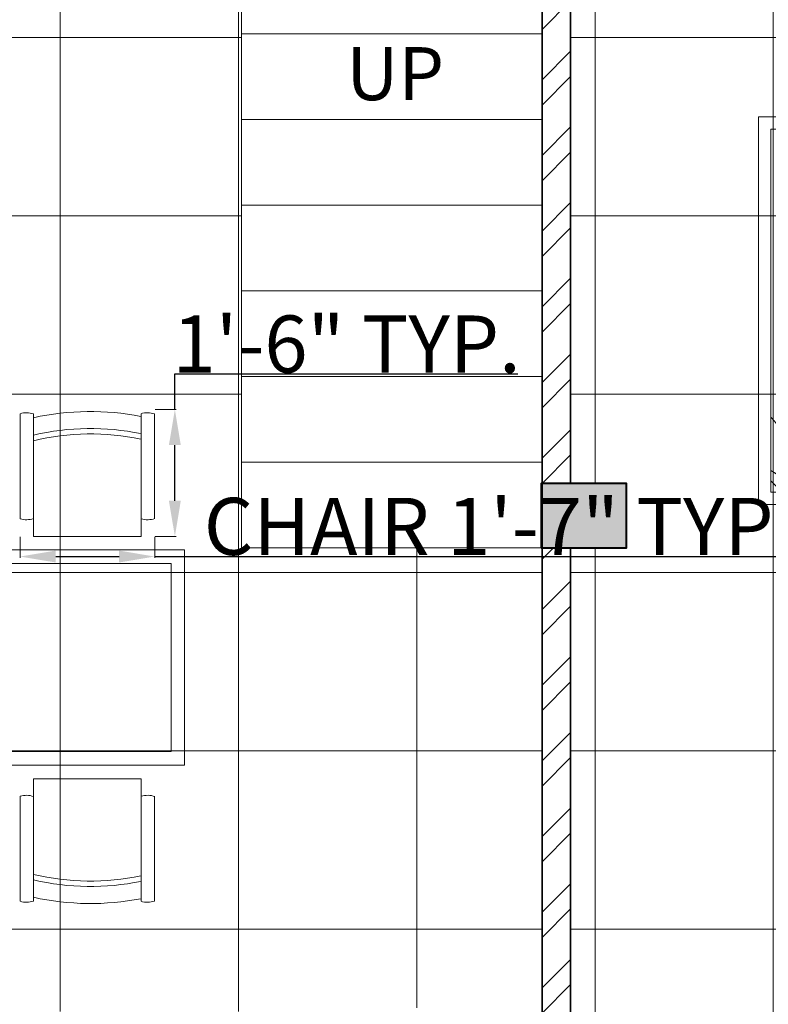
# Model space of a CAD drawing. Units: inches. Extents: x 351 to 1738, y -265 to 286.
# Tile 4 of 38: x 654 to 759, y 0 to 138. Entities that reach past the tile are written whole.
import ezdxf

# ---------------------------------------------------------------- set-up
doc = ezdxf.new("R2010")
doc.units = ezdxf.units.IN
doc.header["$MEASUREMENT"] = 0
for name, color, linetype, lineweight in [('A-ANNO-DIMS', 2, 'Continuous', 18), ('A-ANNO-SYMB', 7, 'Continuous', 18), ('A-COLS', 7, 'Continuous', 40), ('A-COLS-PATT', 6, 'Continuous', 13), ('A-FLOR-PATT', 9, 'Continuous', 9), ('A-FLOR-STRS', 7, 'Continuous', 18), ('A-FURN', 18, 'Continuous', 13), ('A-WALL', 7, 'Continuous', 35), ('A-WALL-PATT', 152, 'Continuous', 13)]:
    doc.layers.add(name, color=color, linetype=linetype, lineweight=lineweight)
doc.styles.add('Annotative', font='arial.ttf')
doc.styles.get("Standard").update_dxf_attribs({"font": 'arial.ttf'})
doc.dimstyles.get("Standard").update_dxf_attribs({"dimtxt": 8, "dimasz": 5, "dimexe": 0.18, "dimexo": 0.0625, "dimgap": 0.09, "dimtad": 1, "dimtoh": 1, "dimzin": 0, "dimdsep": 46, "dimlunit": 4, "dimtxsty": 'Standard', "dimcen": 0, "dimclre": 256, "dimadec": 0, "dimazin": 0, "dimtfac": 1, "dimtofl": 0, "dimtmove": 0, "dimatfit": 3, "dimfxl": 1, "dimtolj": 1, "dimtzin": 0, "dimlwe": -1, "dimarcsym": 0})

# ---------------------------------------------------------------- blocks, each defined once
blk = doc.blocks.new('BED-DOUBLE-W-NIGHTSTANDS')
for p, q in [((30.18, 128.33), (30.18, 86.91)), ((15.09, 105.9), (15.09, 125.61)), ((120.72, 126.39), (30.18, 126.39)), ((135.81, 105.9), (135.81, 125.61)), ((24.95, 115.76), (5.23, 115.76)), ((125.95, 115.76), (145.67, 115.76)), ((30.18, 104.48), (120.72, 104.48)), ((120.32, 98.22), (66.59, 97.46)), ((120.26, 96.67), (65.46, 95.89)), ((120.18, 91.92), (62.88, 91.69)), ((120.19, 90.37), (62.29, 90.13)), ((121.41, 44.95), (28.44, 44.95)), ((121.55, 43.07), (28.44, 43.07)), ((106.08, 28.24), (44.82, 28.24)), ((36.54, 17.05), (36.2, 18.75)), ((47.08, 17.05), (47.42, 18.75)), ((102.76, 17.05), (102.43, 18.75)), ((113.31, 17.05), (113.64, 18.75))]:
    blk.add_line(p, q)
for points in [[(30.18, 103.18), (0, 103.18), (0, 128.33), (150.9, 128.33), (150.9, 103.18), (120.72, 103.18), (120.72, 128.33)], [(16.85, 112.71), (15.09, 115.76), (16.85, 118.81)], [(134.05, 118.81), (135.81, 115.76), (134.05, 112.71)], [(71.64, 104.48), (63.37, 92.97), (60, 84.12), (59.39, 80.15), (54.5, 81.37), (50.53, 83.2), (43.81, 84.12), (36.16, 84.73), (30.05, 84.12), (28.83, 85.34), (34.33, 91.75), (40.14, 96.03), (51.14, 100), (67.6, 104.48)], [(121.56, 54.36), (129.93, 54.36), (129.93, 0), (19.92, 0), (19.92, 54.36), (28.45, 54.36)], [(28.45, 52.61), (21.67, 52.61), (21.67, 1.75), (128.18, 1.75), (128.18, 52.61), (121.53, 52.61)]]:
    blk.add_lwpolyline(points)
for points in [[(38.85, 124.57, 0.074897), (39.03, 114.71, -0.472817)], [(74.74, 114.16, 0.14099), (75.04, 124.22, 0.235245)], [(81.19, 114.16, -0.14099), (80.89, 124.22, -0.235245)], [(112.05, 124.57, -0.074897), (111.87, 114.71, 0.472817)], [(28.51, 71.52, 0.001242), (28.44, 42.89, -0.127202), (25.42, 28.62)], [(121.36, 46.14, 0.056112), (122.46, 37.83, 0.095341), (124.58, 29.84)]]:
    blk.add_lwpolyline(points, format="xyb")
for centre, radius in [((15.09, 115.76), 7.04), ((135.81, 115.76), 7.04), ((15.09, 115.76), 3.52), ((135.81, 115.76), 3.52), ((45.25, 11.58), 0.384), ((104.59, 11.58), 0.384), ((42.74, 7.53), 0.384), ((107.11, 7.53), 0.384)]:
    blk.add_circle(centre, radius)
for centre, radius, start, end in [((122.02, 1560.65), 1438.48, 266.68521, 267.14978), ((59.52, 69.97), 54.73, 82.2196, 99.497), ((71.08, 97.62), 26.89, 81.5249, 103.96), ((82.96, 117.05), 7.46, 63.3437, 106.1026), ((94.14, 98.17), 26.53, 76.3427, 101.1841), ((28.88, 1560.65), 1438.48, 272.85022, 273.31479), ((58.07, 110.76), 19.45, 155.1316, 191.7583), ((92.83, 110.76), 19.45, 348.2417, 24.8684), ((56.95, 109.12), 18.49, 354.0129, 15.8293), ((98.98, 109.12), 18.49, 164.1707, 185.9871), ((44.23, 126.34), 20.22, 255.1039, 281.0369), ((54.88, 140.71), 35.07, 258.0397, 289.2615), ((69.08, 133.05), 26.61, 259.8617, 283.6238), ((83.97, 114.44), 8, 245.0183, 288.5407), ((97.94, 124.85), 19.21, 243.8761, 286.1746), ((106.67, 126.34), 20.22, 258.9631, 284.8961), ((391.24, 86.04), 271.14, 176.1, 180.9282), ((-109.53, 81.59), 138.41, 355.8294, 1.553), ((31.41, 138.78), 56.95, 267.4519, 281.3392), ((45.02, 70.89), 12.28, 66.2616, 101.3392), ((69.87, 137.17), 58.52, 250.1194, 259.3383), ((473.78, 76.18), 353.69, 179.1145, 184.8735), ((59.05, 80.02), 0.364, 268.8623, 19.7536), ((123.44, 29.07), 1.38, 246.5219, 33.8264), ((26.8, 28.72), 1.39, 183.98, 297.3412), ((43.02, -128.84), 157.09, 89.3433, 95.6887), ((26.22, 17.62), 11.42, 33.6671, 63.2997), ((41.52, 24.41), 5.82, 145.785, 184.7304), ((30.41, 27.13), 6.25, 328.8218, 9.1554), ((38.15, 26.57), 1.82, 120.0293, 142.325), ((35.25, 25.5), 4.81, 289.2822, 29.1751), ((37.38, 26.93), 2.26, 311.5653, 23.8354), ((38.15, 26.57), 1.82, 44.4517, 63.558), ((48.37, 25.5), 4.81, 150.8249, 250.7178), ((46.24, 26.93), 2.26, 156.1646, 228.4347), ((45.47, 26.57), 1.82, 113.229, 135.5483), ((45.47, 26.57), 1.82, 37.675, 66.7144), ((42.1, 24.41), 5.82, 355.2696, 34.215), ((53.21, 27.13), 6.25, 169.7133, 211.1782), ((57.4, 17.62), 11.42, 111.4941, 146.3329), ((92.44, 17.62), 11.42, 33.6671, 68.5059), ((107.75, 24.41), 5.82, 145.785, 184.7304), ((96.63, 27.13), 6.25, 328.8218, 10.2867), ((104.38, 26.57), 1.82, 113.2856, 142.325), ((101.48, 25.5), 4.81, 289.2822, 29.1751), ((104.38, 26.57), 1.82, 44.4517, 66.7144), ((103.61, 26.93), 2.26, 311.5653, 23.8354), ((110.71, -118.52), 146.84, 85.2402, 91.8035), ((114.6, 25.5), 4.81, 150.8249, 250.7178), ((112.47, 26.93), 2.26, 156.1646, 228.4347), ((111.7, 26.57), 1.82, 106.6343, 135.5483), ((111.7, 26.57), 1.82, 37.675, 72.5814), ((108.32, 24.41), 5.82, 355.2696, 34.215), ((119.44, 27.13), 6.25, 169.249, 211.1782), ((123.63, 17.62), 11.42, 113.6453, 146.3329), ((34.52, 24.63), 4.34, 7.436, 29.9149), ((49.1, 24.63), 4.34, 150.0851, 172.564), ((100.75, 24.63), 4.34, 7.436, 29.9149), ((115.33, 24.63), 4.34, 150.0851, 172.564), ((32.87, 23.1), 2.55, 84.4856, 181.0538), ((32.09, 21.21), 4.54, 355.2933, 76.921), ((40.93, 22.93), 3.09, 131.5653, 195.1471), ((42.69, 22.93), 3.09, 344.8529, 48.4347), ((51.53, 21.21), 4.54, 103.079, 184.7067), ((50.75, 23.1), 2.55, 358.9462, 95.5144), ((99.1, 23.1), 2.55, 84.4856, 181.0538), ((98.32, 21.21), 4.54, 355.2933, 76.921), ((107.16, 22.93), 3.09, 131.5653, 195.1471), ((108.92, 22.93), 3.09, 344.8529, 48.4347), ((117.76, 21.21), 4.54, 103.079, 184.7067), ((116.98, 23.1), 2.55, 358.9462, 95.5144), ((34.67, 20.3), 3.75, 299.9085, 73.1337), ((48.95, 20.3), 3.75, 106.8663, 240.0915), ((100.89, 20.3), 3.75, 299.9085, 73.1337), ((115.18, 20.3), 3.75, 106.8663, 240.0915), ((33.91, 22.74), 3.61, 174.9449, 262.8857), ((35.33, 24.1), 3.5, 201.5819, 291.4221), ((37.04, 21.88), 0.937, 257.3041, 15.1471), ((46.58, 21.88), 0.937, 164.8529, 282.6959), ((48.29, 24.1), 3.5, 248.5779, 338.4181), ((49.7, 22.74), 3.61, 277.1143, 5.0551), ((100.14, 22.74), 3.61, 174.9449, 262.8857), ((101.56, 24.1), 3.5, 201.5819, 291.4221), ((103.27, 21.88), 0.937, 257.3041, 15.1471), ((112.81, 21.88), 0.937, 164.8529, 282.6959), ((114.52, 24.1), 3.5, 248.5779, 338.4181), ((115.93, 22.74), 3.61, 277.1143, 5.0551), ((33.29, 23.54), 4.38, 272.3591, 324.0401), ((28.53, 21.34), 8.1, 326.2883, 356.5076), ((41.52, 24.41), 5.82, 212.7011, 216.3445), ((42.24, 20.46), 0.291, 102.7051, 280.4384), ((42.21, 20.63), 0.473, 280.4384, 100.4136), ((42.1, 24.41), 5.82, 323.6555, 327.2989), ((50.33, 23.54), 4.38, 215.9599, 267.6409), ((55.09, 21.34), 8.1, 183.4924, 213.7117), ((99.52, 23.54), 4.38, 272.3591, 324.0401), ((94.76, 21.34), 8.1, 326.2883, 356.5076), ((107.75, 24.41), 5.82, 212.7011, 216.3445), ((107.64, 20.63), 0.473, 79.5864, 259.5616), ((107.6, 20.46), 0.291, 259.5616, 77.2949), ((108.32, 24.41), 5.82, 323.6555, 327.2989), ((116.56, 23.54), 4.38, 215.9599, 267.6409), ((121.32, 21.34), 8.1, 183.4924, 213.7117), ((28.59, 21.91), 7.12, 301.2614, 341.7045), ((55.02, 21.91), 7.12, 198.2955, 238.7386), ((76.66, 18.28), 1.63, 63.0274, 163.8037), ((75, 22.1), 3.37, 271.4585, 315.3727), ((78.22, 18.28), 1.63, 16.1963, 116.9726), ((79.87, 22.1), 3.37, 224.6273, 268.5415), ((94.82, 21.91), 7.12, 301.2614, 341.7045), ((121.25, 21.91), 7.12, 198.2955, 238.7386), ((33.08, 16.92), 2.26, 80.264, 250.8688), ((52.7, 12.86), 12.5, 153.0032, 159.8941), ((50.53, 16.92), 2.26, 289.1312, 99.736), ((76.62, -0.91), 19.71, 94.4623, 172.255), ((76.71, 17.27), 2.19, 137.7873, 219.1145), ((74.23, 17.34), 1.65, 298.5391, 58.3627), ((76.37, 15.9), 3.12, 45.5411, 114.3101), ((79.21, 31.89), 13.79, 252.593, 267.2582), ((76.7, 18.68), 1.61, 177.7585, 283.852), ((79.8, 20.35), 4.98, 198.9159, 238.011), ((78.5, 15.9), 3.12, 65.6899, 134.4589), ((75.66, 31.89), 13.79, 272.7418, 287.407), ((75.07, 20.35), 4.98, 301.989, 341.0841), ((78.18, 18.68), 1.61, 256.148, 2.2415), ((80.65, 17.34), 1.65, 121.6373, 241.4609), ((78.17, 17.27), 2.19, 320.8855, 42.2127), ((77.62, 3.64), 15.25, 352.8636, 81.8197), ((99.31, 16.92), 2.26, 80.264, 250.8688), ((97.15, 12.86), 12.5, 20.1059, 26.9968), ((116.76, 16.92), 2.26, 289.1312, 99.736), ((32.54, 17.61), 2.83, 265.969, 344.3045), ((35.59, 13.85), 3.01, 96.1662, 141.5825), ((40.58, 15.96), 0.792, 101.3256, 154.4621), ((39.44, 18.65), 2.39, 280.2588, 300.656), ((38.92, 18.64), 2.42, 308.2101, 316.3071), ((40.41, 17.05), 0.724, 278.3432, 4.2869), ((40.01, 17.68), 1.26, 300.656, 332.6341), ((40.96, 16.85), 0.307, 55.7657, 157.4417), ((41.44, 17.14), 0.307, 84.3784, 186.0543), ((41.15, 18.37), 1.26, 269.1859, 301.164), ((41.52, 17.71), 0.724, 237.5332, 323.4768), ((40.82, 19.78), 2.42, 285.5129, 293.6099), ((42.4, 17.05), 0.792, 87.3579, 140.4944), ((40.57, 19.33), 2.39, 301.164, 321.5612), ((38.63, 19.74), 4.26, 324.6898, 333.4936), ((48.03, 13.85), 3.01, 38.4175, 83.8338), ((51.08, 17.61), 2.83, 195.6955, 274.031), ((77.04, 17.32), 0.213, 283.852, 219.9245), ((77.29, 16.34), 0.245, 238.011, 71.5592), ((77.33, 16.45), 0.119, 71.5592, 188.0167), ((77.58, 16.34), 0.245, 108.4408, 301.989), ((77.54, 16.45), 0.119, 351.9833, 108.4408), ((77.82, 17.4), 0.128, 320.1909, 256.0209), ((98.77, 17.61), 2.83, 265.969, 344.3045), ((101.82, 13.85), 3.01, 96.1662, 141.5825), ((109.28, 19.33), 2.39, 218.4388, 238.836), ((107.45, 17.05), 0.792, 39.5056, 92.6421), ((111.22, 19.74), 4.26, 206.5064, 215.3102), ((108.33, 17.71), 0.724, 216.5232, 302.4668), ((108.7, 18.37), 1.26, 238.836, 270.8141), ((109.03, 19.78), 2.42, 246.3901, 254.4871), ((108.41, 17.14), 0.307, 353.9457, 95.6216), ((109.44, 17.05), 0.724, 175.7131, 261.6568), ((108.89, 16.85), 0.307, 22.5583, 124.2343), ((109.84, 17.68), 1.26, 207.3659, 239.344), ((110.93, 18.64), 2.42, 223.6929, 231.7899), ((110.41, 18.65), 2.39, 239.344, 259.7412), ((109.27, 15.96), 0.792, 25.5379, 78.6744), ((117.31, 17.61), 2.83, 195.6955, 274.031), ((114.26, 13.85), 3.01, 38.4175, 83.8338), ((31.17, 13.79), 1.63, 92.9516, 193.728), ((27.83, 16.28), 3.37, 301.3827, 345.2969), ((32.62, 14.47), 1.39, 63.9755, 143.2681), ((38.45, 14.92), 0.297, 345.2356, 144.9248), ((39.99, 20.56), 4.26, 268.3264, 277.1302), ((52.7, 12.86), 12.5, 163.5842, 183.8277), ((51, 14.47), 1.39, 36.7319, 116.0245), ((52.45, 13.79), 1.63, 346.272, 87.0484), ((55.79, 16.28), 3.37, 194.7031, 238.6173), ((97.39, 13.79), 1.63, 92.9516, 193.728), ((94.06, 16.28), 3.37, 301.3827, 345.2969), ((98.85, 14.47), 1.39, 63.9755, 143.2681), ((97.15, 12.86), 12.5, 356.1723, 16.4158), ((109.86, 20.56), 4.26, 262.8698, 271.6736), ((111.4, 14.92), 0.297, 35.0752, 194.7644), ((117.23, 14.47), 1.39, 36.7319, 116.0245), ((122.02, 16.28), 3.37, 194.7031, 238.6173), ((118.68, 13.79), 1.63, 346.272, 87.0484), ((32.11, 11.59), 3.12, 75.4653, 144.2343), ((26.59, 26.86), 13.79, 282.5173, 297.1824), ((38.34, 14.46), 0.641, 101.5637, 142.6358), ((37.8, 13.86), 0.384, 273.2768, 86.7232), ((38.25, 14.23), 0.367, 91.1081, 181.8675), ((38.64, 13.49), 0.794, 80.3487, 133.6538), ((37.82, 14.96), 0.924, 288.7263, 352.5032), ((38.49, 12.66), 1.26, 83.0852, 105.7171), ((38.72, 13.95), 0.331, 317.6792, 80.3487), ((51.51, 11.59), 3.12, 35.7657, 104.5347), ((57.03, 26.86), 13.79, 242.8176, 257.4827), ((98.34, 11.59), 3.12, 75.4653, 144.2343), ((92.82, 26.86), 13.79, 282.5173, 297.1824), ((111.13, 13.95), 0.331, 99.6513, 222.3208), ((111.21, 13.49), 0.794, 46.3462, 99.6513), ((112.03, 14.96), 0.924, 187.4968, 251.2737), ((111.36, 12.66), 1.26, 74.2829, 96.9148), ((111.6, 14.23), 0.367, 358.1325, 88.8919), ((111.51, 14.46), 0.641, 37.3642, 78.4363), ((112.04, 13.86), 0.384, 93.2768, 266.7232), ((117.74, 11.59), 3.12, 35.7657, 104.5347), ((123.26, 26.86), 13.79, 242.8176, 257.4827), ((40.71, -2.86), 19.71, 124.3865, 158.5908), ((31.71, 12.94), 2.19, 167.7115, 249.0387), ((29.53, 11.76), 1.65, 328.4633, 88.2869), ((32.86, 17.16), 4.98, 228.8402, 267.9352), ((31.01, 14.16), 1.61, 207.6827, 313.7762), ((31.97, 13.15), 0.213, 313.7762, 249.7183), ((32.66, 12.55), 0.119, 101.4834, 217.9409), ((32.69, 12.42), 0.245, 267.9352, 101.4834), ((38.33, 13.15), 0.634, 217.7621, 259.0403), ((39.01, 14), 1.17, 203.4276, 227.6104), ((38.5, 14.15), 0.629, 229.7889, 317.6792), ((37.79, 12.81), 0.893, 355.053, 68.3618), ((38.39, 12.76), 0.295, 232.4737, 355.053), ((29.78, 2.23), 14.33, 43.1541, 52.0459), ((42.31, 12.15), 1.75, 304.5369, 16.3699), ((44.74, 11.66), 1.24, 127.3105, 187.9252), ((43.04, 11.8), 1.27, 355.0106, 41.658), ((44.83, 12.11), 0.524, 126.1046, 271.4281), ((44.77, 12.26), 0.377, 353.7526, 131.7054), ((45.79, 12.17), 0.641, 101.5637, 176.365), ((45.27, 12.68), 0.924, 288.7263, 352.5032), ((45.9, 12.63), 0.297, 345.2356, 144.9248), ((50.93, 12.42), 0.245, 78.5166, 272.0648), ((50.76, 17.16), 4.98, 272.0648, 311.1598), ((50.96, 12.55), 0.119, 322.0591, 78.5166), ((52.61, 14.16), 1.61, 226.2238, 332.3173), ((51.67, 13.23), 0.128, 290.2667, 226.2271), ((54.09, 11.76), 1.65, 91.7131, 211.5367), ((51.9, 12.94), 2.19, 290.9613, 12.2885), ((42.91, -2.86), 19.71, 21.4092, 55.6135), ((106.94, -2.86), 19.71, 124.3865, 158.5908), ((97.94, 12.94), 2.19, 167.7115, 249.0387), ((97.24, 14.16), 1.61, 207.6827, 313.7762), ((99.09, 17.16), 4.98, 228.8402, 267.9352), ((95.76, 11.76), 1.65, 328.4633, 88.2869), ((98.2, 13.15), 0.213, 313.7762, 249.7183), ((98.89, 12.55), 0.119, 101.4834, 217.9409), ((98.92, 12.42), 0.245, 267.9352, 101.4834), ((103.95, 12.63), 0.297, 35.0752, 194.7644), ((104.58, 12.68), 0.924, 187.4968, 251.2737), ((104.06, 12.17), 0.641, 3.635, 78.4363), ((105.08, 12.26), 0.377, 48.2946, 186.2474), ((105.02, 12.11), 0.524, 268.5719, 53.8954), ((106.81, 11.8), 1.27, 138.342, 184.9894), ((107.53, 12.15), 1.75, 163.6301, 235.4631), ((105.1, 11.66), 1.24, 352.0748, 52.6895), ((120.07, 2.23), 14.33, 127.9541, 136.8459), ((111.35, 14.15), 0.629, 222.3208, 310.2111), ((112.06, 12.81), 0.893, 111.6382, 184.947), ((111.46, 12.76), 0.295, 184.947, 307.5263), ((110.83, 14), 1.17, 312.3896, 336.5724), ((111.52, 13.15), 0.634, 280.9597, 322.2379), ((117.16, 12.42), 0.245, 78.5166, 272.0648), ((116.99, 17.16), 4.98, 272.0648, 311.1598), ((117.18, 12.55), 0.119, 322.0591, 78.5166), ((118.84, 14.16), 1.61, 226.2238, 332.3173), ((117.9, 13.23), 0.128, 290.2667, 226.2271), ((120.32, 11.76), 1.65, 91.7131, 211.5367), ((118.13, 12.94), 2.19, 290.9613, 12.2885), ((109.14, -2.86), 19.71, 21.4092, 55.6135), ((7, -0.91), 19.71, 7.745, 41.8856), ((39.68, 10.88), 0.792, 101.3256, 154.4621), ((38.54, 13.57), 2.39, 280.2588, 300.656), ((39.09, 15.48), 4.26, 268.3264, 277.1302), ((38.02, 13.56), 2.42, 308.2101, 316.3071), ((39.51, 11.97), 0.724, 278.3432, 4.2869), ((39.11, 12.61), 1.26, 300.656, 332.6341), ((40.06, 11.77), 0.307, 55.7657, 157.4417), ((46.48, 12.55), 6.27, 184.756, 209.2041), ((55.5, 25.89), 20.62, 222.2412, 232.1744), ((43.25, 11.76), 1.06, 272.8499, 356.1226), ((42.5, 11.35), 1.03, 321.7607, 7.9252), ((44.45, 10.86), 0.381, 148.0499, 225.6268), ((47.12, 4.22), 7.52, 113.0501, 113.8477), ((45.15, 10.42), 1.21, 104.7558, 148.0499), ((44.47, 11.29), 0.758, 247.4086, 351.4386), ((44.68, 11.26), 0.255, 262.906, 7.132), ((44.42, 11.81), 0.529, 0.0645, 61.1507), ((44.54, 12.26), 0.604, 311.8413, 355.7877), ((45.78, 10.87), 0.634, 151.2196, 259.0403), ((45.7, 11.94), 0.367, 91.1081, 181.8675), ((46.46, 11.71), 1.17, 203.4276, 227.6104), ((46.09, 11.2), 0.794, 80.3487, 133.6538), ((45.95, 11.86), 0.629, 229.7889, 317.6792), ((45.24, 10.53), 0.893, 355.053, 68.3618), ((45.94, 10.38), 1.26, 83.0852, 105.7171), ((46.17, 11.66), 0.331, 317.6792, 80.3487), ((47.12, 4.22), 7.52, 87.1071, 94.7585), ((102.73, 4.22), 7.52, 85.2415, 92.8929), ((103.68, 11.66), 0.331, 99.6513, 222.3208), ((103.9, 11.86), 0.629, 222.3208, 310.2111), ((103.76, 11.2), 0.794, 46.3462, 99.6513), ((104.61, 10.53), 0.893, 111.6382, 184.947), ((103.91, 10.38), 1.26, 74.2829, 96.9148), ((104.15, 11.94), 0.367, 358.1325, 88.8919), ((103.38, 11.71), 1.17, 312.3896, 336.5724), ((104.07, 10.87), 0.634, 280.9597, 28.7804), ((105.38, 11.29), 0.758, 188.5614, 292.5914), ((105.3, 12.26), 0.604, 184.2123, 228.1587), ((105.43, 11.81), 0.529, 118.8493, 179.9355), ((105.16, 11.26), 0.255, 172.868, 277.094), ((104.7, 10.42), 1.21, 31.9501, 75.2442), ((106.6, 11.76), 1.06, 183.8774, 267.1501), ((102.73, 4.22), 7.52, 66.1523, 66.9499), ((105.4, 10.86), 0.381, 314.3732, 31.9501), ((107.35, 11.35), 1.03, 172.0748, 218.2393), ((94.35, 25.89), 20.62, 307.8256, 317.7588), ((103.37, 12.55), 6.27, 330.7959, 355.244), ((110.34, 11.97), 0.724, 175.7131, 261.6568), ((109.79, 11.77), 0.307, 22.5583, 124.2343), ((110.74, 12.61), 1.26, 207.3659, 239.344), ((111.83, 13.56), 2.42, 223.6929, 231.7899), ((111.31, 13.57), 2.39, 239.344, 259.7412), ((110.76, 15.48), 4.26, 262.8698, 271.6736), ((110.17, 10.88), 0.792, 25.5379, 78.6744), ((142.85, -0.91), 19.71, 138.1144, 172.255), ((39.94, 9.49), 0.429, 146.8636, 236.9021), ((45.99, 18.94), 11.23, 235.1882, 238.8844), ((40.68, 10.11), 1.16, 199.4799, 267.6828), ((47.12, 4.22), 7.52, 120.544, 139.818), ((42.71, 9.86), 1.03, 8.7227, 54.8872), ((42.77, 9.04), 1.75, 0.278, 72.111), ((43.55, 9.68), 1.06, 20.5253, 88.5375), ((44.96, 10.21), 1.24, 188.7227, 249.3375), ((43.37, 9.59), 1.27, 334.9899, 21.6373), ((45.84, 10.48), 0.295, 232.4737, 355.053), ((104.01, 10.48), 0.295, 184.947, 307.5263), ((106.48, 9.59), 1.27, 158.3627, 205.0101), ((106.3, 9.68), 1.06, 91.4625, 159.4747), ((107.08, 9.04), 1.75, 107.889, 179.722), ((104.89, 10.21), 1.24, 290.6625, 351.2773), ((107.13, 9.86), 1.03, 125.1128, 171.2773), ((102.73, 4.22), 7.52, 40.182, 59.456), ((109.17, 10.11), 1.16, 272.3172, 340.5201), ((103.85, 18.94), 11.23, 301.1156, 304.8118), ((109.9, 9.49), 0.429, 303.0979, 33.1364), ((40.55, 9.68), 1, 212.8155, 277.3992), ((39.97, 9.01), 1.16, 266.9701, 338.2913), ((40.42, 9.71), 0.444, 238.8844, 314.2646), ((40.33, 8.72), 1, 280.3057, 17.1958), ((40.24, 8.61), 0.444, 306.3746, 21.7548), ((40.96, 8.9), 0.335, 19.3605, 201.7548), ((40.97, 9.16), 0.335, 311.8703, 134.2646), ((47.27, 6.1), 6.69, 153.7819, 158.2913), ((41.94, 10.67), 1.75, 247.2305, 319.0635), ((41.36, 10.08), 1.03, 264.4544, 310.6188), ((46.48, 12.55), 6.27, 214.0033, 222.4917), ((42.12, 9.68), 1.06, 218.3208, 298.8162), ((42.32, 8.06), 0.524, 126.1046, 271.4281), ((42.26, 8.21), 0.377, 353.7526, 131.7054), ((42.84, 8.36), 1.24, 70.0041, 130.6188), ((42.04, 9.87), 1.27, 297.7043, 344.3516), ((43.27, 8.12), 0.641, 101.5637, 176.365), ((42.76, 8.63), 0.924, 288.7263, 352.5032), ((43.39, 8.58), 0.297, 345.2356, 144.9248), ((75.15, 7.73), 1.63, 63.0274, 163.8037), ((73.5, 11.55), 3.37, 271.4585, 315.3727), ((74.86, 5.35), 3.12, 45.5411, 114.3101), ((80.01, 5.35), 3.12, 65.6899, 134.4589), ((79.73, 7.73), 1.63, 16.1963, 116.9726), ((81.38, 11.55), 3.37, 224.6273, 268.5415), ((106.46, 8.58), 0.297, 35.0752, 194.7644), ((107.09, 8.63), 0.924, 187.4968, 251.2737), ((107.01, 8.36), 1.24, 49.3812, 109.9959), ((107.91, 10.67), 1.75, 220.9365, 292.7695), ((107.81, 9.87), 1.27, 195.6484, 242.2957), ((106.58, 8.12), 0.641, 3.635, 78.4363), ((107.59, 8.21), 0.377, 48.2946, 186.2474), ((107.73, 9.68), 1.06, 241.1838, 321.6792), ((107.53, 8.06), 0.524, 268.5719, 53.8954), ((108.49, 10.08), 1.03, 229.3812, 275.5456), ((103.37, 12.55), 6.27, 317.5083, 325.9967), ((109.52, 8.72), 1, 162.8042, 259.6943), ((108.88, 9.16), 0.335, 45.7354, 228.1297), ((108.88, 8.9), 0.335, 338.2452, 160.6395), ((102.58, 6.1), 6.69, 21.7087, 26.2181), ((109.88, 9.01), 1.16, 201.7087, 273.0299), ((109.42, 9.71), 0.444, 225.7354, 301.1156), ((109.61, 8.61), 0.444, 158.2452, 233.6254), ((109.3, 9.68), 1, 262.6008, 327.1845), ((33.85, 17.3), 11.23, 302.6784, 306.3746), ((40.26, 8.09), 0.429, 214.3538, 304.3923), ((41.93, 6.81), 0.381, 148.0499, 225.6268), ((42.64, 6.37), 1.21, 104.7558, 148.0499), ((41.96, 7.24), 0.758, 247.4086, 351.4386), ((42.17, 7.2), 0.255, 262.906, 7.132), ((41.9, 7.76), 0.529, 0.0645, 61.1507), ((42.03, 8.21), 0.604, 311.8413, 355.7877), ((43.26, 6.82), 0.634, 151.2196, 259.0403), ((43.19, 7.89), 0.367, 91.1081, 181.8675), ((43.95, 7.66), 1.17, 203.4276, 227.6104), ((43.58, 7.15), 0.794, 80.3487, 133.6538), ((43.44, 7.81), 0.629, 229.7889, 317.6792), ((42.73, 6.48), 0.893, 355.053, 68.3618), ((43.43, 6.33), 1.26, 83.0852, 105.7171), ((43.66, 7.61), 0.331, 317.6792, 80.3487), ((75.11, -11.46), 19.71, 94.4623, 117.4146), ((75.2, 6.72), 2.19, 137.7873, 219.1145), ((72.72, 6.78), 1.65, 298.5391, 58.3627), ((78.3, 9.8), 4.98, 198.9159, 238.011), ((77.71, 21.34), 13.79, 252.593, 267.2582), ((75.19, 8.12), 1.61, 177.7585, 283.852), ((75.53, 6.76), 0.213, 283.852, 219.9245), ((77.17, 21.34), 13.79, 272.7418, 287.407), ((79.33, 6.85), 0.128, 320.1909, 256.0209), ((76.58, 9.8), 4.98, 301.989, 341.0841), ((79.69, 8.12), 1.61, 256.148, 2.2415), ((82.16, 6.78), 1.65, 121.6373, 241.4609), ((79.68, 6.72), 2.19, 320.8855, 42.2127), ((79.76, -11.46), 19.71, 62.5854, 85.5377), ((106.19, 7.61), 0.331, 99.6513, 222.3208), ((106.41, 7.81), 0.629, 222.3208, 310.2111), ((106.27, 7.15), 0.794, 46.3462, 99.6513), ((107.12, 6.48), 0.893, 111.6382, 184.947), ((106.42, 6.33), 1.26, 74.2829, 96.9148), ((106.66, 7.89), 0.367, 358.1325, 88.8919), ((105.9, 7.66), 1.17, 312.3896, 336.5724), ((106.58, 6.82), 0.634, 280.9597, 28.7804), ((107.89, 7.24), 0.758, 188.5614, 292.5914), ((107.82, 8.21), 0.604, 184.2123, 228.1587), ((107.94, 7.76), 0.529, 118.8493, 179.9355), ((107.68, 7.2), 0.255, 172.868, 277.094), ((107.21, 6.37), 1.21, 31.9501, 75.2442), ((107.91, 6.81), 0.381, 314.3732, 31.9501), ((116, 17.3), 11.23, 233.6254, 237.3216), ((109.59, 8.09), 0.429, 235.6077, 325.6462), ((43.32, 6.43), 0.295, 232.4737, 355.053), ((66.74, -3.55), 9.6, 91.272, 146.5383), ((70.19, -5.34), 11.97, 107.8504, 143.6964), ((76.48, -8.7), 17.8, 124.0123, 144.053), ((75.79, 5.78), 0.245, 238.011, 71.5592), ((75.83, 5.9), 0.119, 71.5592, 188.0167), ((79.09, 5.78), 0.245, 108.4408, 301.989), ((79.05, 5.9), 0.119, 351.9833, 108.4408), ((79.59, 5.04), 8.82, 338.117, 6.6195), ((87.68, 2.58), 3.54, 346.3898, 79.0739), ((85.02, 3.07), 4.47, 342.8609, 41.9049), ((106.52, 6.43), 0.295, 184.947, 307.5263), ((16.88, -3.55), 9.6, 33.4617, 60.1116), ((22.26, -1.32), 8.01, 22.5547, 48.9546), ((0.31, 2.98), 27.26, 357.4081, 3.6519), ((61.36, -1.32), 8.01, 131.0454, 157.4453), ((83.31, 2.98), 27.26, 176.3481, 182.5919), ((66.54, 2.98), 27.26, 357.4081, 3.6519), ((88.49, -1.32), 8.01, 22.5547, 48.9546), ((127.59, -1.32), 8.01, 131.0454, 157.4453), ((149.54, 2.98), 27.26, 176.3481, 182.5919), ((132.97, -3.55), 9.6, 119.8884, 146.5383), ((13.43, -5.34), 11.97, 36.3036, 46.4814), ((136.42, -5.34), 11.97, 133.5186, 143.6964), ((69.6, -8.61), 10.84, 73.5431, 107.0202), ((73.9, -14.2), 16.02, 94.3787, 95.6357), ((82.34, -25.17), 28.63, 109.7217, 109.9028), ((85.27, -8.61), 10.84, 72.9798, 106.4569), ((80.98, -14.2), 16.02, 84.3643, 85.6213), ((72.54, -25.17), 28.63, 70.0972, 70.2783)]:
    blk.add_arc(centre, radius, start, end)
blk = doc.blocks.new('CHAIR-DINING')
for p, q in [((0, 2.47), (0, 17.19)), ((18.84, 17.16), (18.84, 2.49))]:
    blk.add_line(p, q)
blk.add_lwpolyline([(16.96, 17.18), (16.96, 0), (1.88, 0), (1.88, 17.15)])
for centre, radius, start, end in [((0.89, 14.39), 2.93, 70.2624, 107.7226), ((9.88, -19.57), 37.07, 78.9982, 102.4562), ((17.86, 14.39), 2.93, 70.4535, 107.9116), ((9.88, -20.08), 35.19, 78.4012, 103.1346), ((9.88, -20.08), 34.43, 78.1438, 103.4274), ((0.89, 5.26), 2.93, 252.2774, 289.7376), ((17.89, 5.26), 2.93, 252.2774, 289.7376)]:
    blk.add_arc(centre, radius, start, end)
blk = doc.blocks.new('COL-9x12')
blk.add_lwpolyline([(0, 12), (0, 0), (9, 0), (9, 12)], close=True)
blk = doc.blocks.new('*D40')
at = {"layer": 'A-ANNO-DIMS', "transparency": 16777216}
for p, q in [((654.45, 65.99), (654.45, 63.04)), ((673.33, 65.99), (673.33, 63.04))]:
    blk.add_line(p, q, dxfattribs=at)
at = {"layer": 'A-ANNO-DIMS', "color": 0, "lineweight": -2, "transparency": 16777216}
for p, q in [((659.45, 63.22), (668.33, 63.22)), ((673.33, 63.22), (765.05, 63.22))]:
    blk.add_line(p, q, dxfattribs=at)
at = {"layer": 'A-ANNO-DIMS', "color": 0, "transparency": 16777216}
for points in [[(659.45, 64.06), (659.45, 62.39), (654.45, 63.22)], [(668.33, 64.06), (668.33, 62.39), (673.33, 63.22)]]:
    blk.add_solid(points, dxfattribs=at)
at = {"layer": 'Defpoints', "color": 0, "transparency": 16777216}
for p in [(654.45, 66.05), (673.33, 66.05), (673.33, 63.22)]:
    blk.add_point(p, dxfattribs=at)
at = {"layer": 'A-ANNO-DIMS', "color": 0, "transparency": 16777216, "insert": (721.69, 67.45), "char_height": 8, "attachment_point": 5}
blk.add_mtext('\\A1;CHAIR 1\'-7" TYP.', dxfattribs=at)
blk = doc.blocks.new('*D41')
at = {"layer": 'A-ANNO-DIMS', "color": 0, "lineweight": -2, "transparency": 16777216}
for p, q in [((676.16, 83.84), (676.16, 88.84)), ((676.16, 88.84), (724.26, 88.84)), ((676.16, 71.05), (676.16, 78.84))]:
    blk.add_line(p, q, dxfattribs=at)
at = {"layer": 'A-ANNO-DIMS', "transparency": 16777216}
for p, q in [((673.39, 83.84), (676.34, 83.84)), ((673.39, 66.05), (676.34, 66.05))]:
    blk.add_line(p, q, dxfattribs=at)
at = {"layer": 'A-ANNO-DIMS', "color": 0, "transparency": 16777216}
for points in [[(675.32, 78.84), (676.99, 78.84), (676.16, 83.84)], [(675.32, 71.05), (676.99, 71.05), (676.16, 66.05)]]:
    blk.add_solid(points, dxfattribs=at)
at = {"layer": 'Defpoints', "color": 0, "transparency": 16777216}
for p in [(673.33, 83.84), (676.16, 83.84), (673.33, 66.05)]:
    blk.add_point(p, dxfattribs=at)
at = {"layer": 'A-ANNO-DIMS', "color": 0, "transparency": 16777216, "insert": (700.25, 93.01), "char_height": 8, "attachment_point": 5}
blk.add_mtext('\\A1;1\'-6" TYP.', dxfattribs=at)

msp = doc.modelspace()

# ---------------------------------------------------------------- hatches: boundary and pattern name
at = {"layer": 'A-COLS-PATT'}
h = msp.add_hatch(color=256, dxfattribs=at)
h.dxf.hatch_style = 1
h.paths.add_polyline_path([(460.155, 237.963), (451.155, 237.963), (451.155, 228.963), (460.155, 228.963)])
h.paths.add_polyline_path([(463.155, 237.963), (460.155, 237.963), (460.155, 228.963), (463.155, 228.963)])
h.paths.add_polyline_path([(391.155, 255.963), (382.155, 255.963), (382.155, 243.963), (391.155, 243.963)])
h.paths.add_polyline_path([(391.155, 210.963), (382.155, 210.963), (382.155, 198.963), (391.155, 198.963)])
h.paths.add_polyline_path([(391.155, -45.037), (382.155, -45.037), (382.155, -57.037), (391.155, -57.037)])
h.paths.add_polyline_path([(460.155, -45.037), (451.155, -45.037), (451.155, -57.037), (460.155, -57.037)])
h.paths.add_polyline_path([(460.155, -161.037), (451.155, -161.037), (451.155, -164.037), (451.155, -173.037), (460.155, -173.037)])
h.paths.add_polyline_path([(391.155, -161.037), (382.155, -161.037), (382.155, -173.037), (391.155, -173.037)])
h.paths.add_polyline_path([(596, -164.037), (584, -164.037), (584, -173.037), (596, -173.037)])
h.paths.add_polyline_path([(596, -50), (584, -50), (584, -59), (596, -59)])
h.paths.add_polyline_path([(596.155, 73.463), (592.155, 73.463), (592.155, 64.463), (596.155, 64.463)])
h.paths.add_polyline_path([(592.155, 73.463), (584.155, 73.463), (584.155, 64.463), (592.155, 64.463)])
h.paths.add_polyline_path([(596.155, 237.963), (584.155, 237.963), (584.155, 228.963), (596.155, 228.963)])
h.paths.add_polyline_path([(739.655, 237.963), (727.655, 237.963), (727.655, 228.963), (739.655, 228.963)])
h.paths.add_polyline_path([(883.515, 237.963), (871.515, 237.963), (871.515, 228.963), (883.515, 228.963)])
h.paths.add_polyline_path([(883.515, 73.463), (871.515, 73.463), (871.515, 64.463), (883.515, 64.463)])
h.paths.add_polyline_path([(731.655, 73.463), (727.655, 73.463), (727.655, 64.463), (731.655, 64.463)])
h.paths.add_polyline_path([(739.515, 73.463), (731.655, 73.463), (731.655, 64.463), (739.515, 64.463)])
h.paths.add_polyline_path([(883.515, -53.037), (871.515, -53.037), (871.515, -57.037), (883.515, -57.037)])
h.paths.add_polyline_path([(883.515, -48.037), (871.515, -48.037), (871.515, -53.037), (883.515, -53.037)])
h.paths.add_polyline_path([(739.515, -48.037), (727.515, -48.037), (727.515, -56.5), (727.516, -57.037), (739.515, -57.037)])
h.paths.add_polyline_path([(883.515, -164.037), (871.515, -164.037), (871.515, -173.037), (883.515, -173.037)])
at = {"layer": 'A-FLOR-PATT', "transparency": 33554559}
h = msp.add_hatch(dxfattribs=at)
h.set_pattern_fill('ANSI37', color=256, scale=200, angle=45)
h.set_pattern_definition([(90, (460.077, -164.037), (-25, 0), []), (180, (460.077, -164.037), (-4e-15, -25), [])])
h.paths.add_polyline_path([(727.516, -57.037), (727.515, -57.037), (727.515, -56.5), (727.5, -45), (727.5, -3.5), (727.501, -2.537), (725.797, -2.537), (725.797, -3.037), (721.988, -3.037), (721.988, -2.537), (717.916, -2.537), (717.916, -3.037), (714.106, -3.037), (714.106, -2.537), (710.487, -2.537), (710.487, -3.037), (706.677, -3.037), (706.677, -2.537), (702.965, -2.537), (702.965, -3.037), (699.155, -3.037), (699.155, -2.537), (694.965, -2.537), (694.965, -3.037), (691.155, -3.037), (691.155, -2.537), (679.655, -2.537), (678.797, -2.537), (677.776, -2.537), (676.723, -2.537), (652.655, -2.537), (651.799, -2.537), (650.778, -2.537), (649.725, -2.537), (625.877, -2.537), (624.879, -2.537), (623.857, -2.537), (622.804, -2.537), (596.155, -2.537), (596.155, -3.537), (460.155, -3.537), (460.155, -81.037), (460.077, -99.07), (460.077, -133.967), (460.155, -152.037), (460.155, -164.037), (485.277, -164.037), (545.277, -164.037), (727.655, -164.037)])
h.paths.add_polyline_path([(584, -59), (584, -50), (596, -50), (596, -59)], flags=16)
h.paths.add_polyline_path([(905.155, 204.963), (731.655, 204.963), (731.655, 73.463), (739.515, 73.463), (739.515, 64.463), (731.655, 64.463), (731.655, -3.5), (727.655, -3.5), (727.655, -3.537), (727.5, -45), (731.655, -45), (731.655, -48.037), (739.515, -48.037), (739.515, -53.037), (754, -53.037), (754, -57.037), (748.655, -57.037), (748.655, -147.037), (815.655, -147.037), (815.655, -138.5), (819.655, -138.5), (819.655, -102.5), (815.655, -102.5), (815.655, -57.037), (790, -57.037), (790, -53.037), (871.515, -53.037), (871.515, -48.037), (883.515, -48.037), (883.515, -53.037), (905.155, -53.037)])
h.paths.add_polyline_path([(871.515, 64.463), (871.515, 73.463), (883.515, 73.463), (883.515, 64.463)], flags=16)
h.paths.add_polyline_path([(727.655, 64.463), (685.515, 64.463), (685.515, 186.963), (638.155, 186.963), (638.155, 88.463), (596.155, 88.463), (596.155, 64.463), (584.155, 64.463), (584.155, 73.463), (592.155, 73.463), (592.155, 205.963), (574, 205.963), (574, 209.963), (538, 209.963), (538, 205.963), (536.5, 205.963), (536.5, 180), (489.5, 180), (489.5, 68.655), (460.155, 68.655), (460.155, 64.463), (536.155, 64.463), (536.155, 48.463), (532.155, 48.463), (532.155, 60.463), (460.155, 60.463), (460.155, 0.463), (532.155, 0.463), (532.155, 12.463), (536.155, 12.463), (536.155, 0.463), (596.155, 0.463), (596.155, -0.537), (622.655, -0.537), (623.655, -0.537), (624.655, -0.537), (625.655, -0.537), (649.655, -0.537), (650.576, -0.537), (651.576, -0.537), (652.576, -0.537), (676.655, -0.537), (677.574, -0.537), (678.574, -0.537), (679.574, -0.537), (691.155, -0.537), (691.155, -0.037), (694.965, -0.037), (694.965, -0.537), (699.155, -0.537), (699.155, -0.037), (702.965, -0.037), (702.965, -0.537), (706.677, -0.537), (706.677, -0.037), (710.487, -0.037), (710.487, -0.537), (714.106, -0.537), (714.106, -0.037), (717.916, -0.037), (717.916, -0.537), (721.988, -0.537), (721.988, -0.037), (725.797, -0.037), (725.797, -0.537), (727.655, -0.537)])
h.paths.add_polyline_path([(485.401, 6.538), (461.783, 6.538), (461.783, 51.327), (485.401, 51.327)], flags=16)
h.paths.add_polyline_path([(483.401, 8.538), (463.783, 8.538), (463.783, 49.327), (483.401, 49.327)], flags=0)
h.paths.add_polyline_path([(476.907, 30.5), (476.907, 29.5), (476.907, 26), (475.907, 26), (475.907, 29.5), (474.449, 29.5), (474.449, 26), (473.449, 26), (470.5, 26), (470.5, 27), (473.449, 27), (473.449, 29.5), (470.5, 29.5), (470.5, 32.758), (471.5, 32.758), (471.5, 30.5), (473.407, 30.5), (473.407, 32.897), (473.407, 33.897), (476.907, 33.897), (476.907, 32.897), (474.407, 32.897), (474.407, 30.5)], flags=0)
at = {"layer": 'A-WALL-PATT'}
h = msp.add_hatch(dxfattribs=at)
h.set_pattern_fill('ANSI32', color=256, scale=20)
h.set_pattern_definition([(45, (382.155, -173.037), (-5.3033, 5.3033), []), (45, (385.691, -173.037), (-5.3033, 5.3033), [])])
h.paths.add_polyline_path([(391.155, -57.037), (382.155, -57.037), (382.155, -81.037), (391.155, -81.037)])
h.paths.add_polyline_path([(391.155, 198.963), (382.155, 198.963), (382.155, -45.037), (391.155, -45.037)])
h.paths.add_polyline_path([(391.155, 243.963), (382.155, 243.963), (382.155, 237.963), (382.155, 210.963), (391.155, 210.963)])
h.paths.add_polyline_path([(460.155, 255.963), (391.155, 255.963), (391.155, 246.963), (451.155, 246.963), (451.155, 237.963), (460.155, 237.963), (460.155, 251.963)])
h.paths.add_polyline_path([(404.155, 207.963), (391.155, 207.963), (391.155, 198.963), (404.155, 198.963)])
h.paths.add_polyline_path([(451.155, 207.963), (440.155, 207.963), (440.155, 198.963), (451.155, 198.963)])
h.paths.add_polyline_path([(460.155, 228.963), (451.155, 228.963), (451.155, 74.963), (460.155, 74.963), (460.155, 97.5)])
h.paths.add_polyline_path([(460.155, 60.463), (532.155, 60.463), (532.155, 48.463), (536.155, 48.463), (536.155, 64.463), (460.155, 64.463), (460.155, 62.963), (451.155, 62.963), (451.155, 46.258), (460.155, 46.258)])
h.paths.add_polyline_path([(460.155, -3.537), (596.155, -3.537), (596.155, 0.463), (536.155, 0.463), (536.155, 12.463), (532.155, 12.463), (532.155, 0.463), (460.155, 0.463), (460.155, 10.258), (451.155, 10.258), (451.155, -45.037), (460.155, -45.037)])
h.paths.add_polyline_path([(460.155, -57.037), (451.155, -57.037), (451.155, -81.037), (460.155, -81.037)])
h.paths.add_polyline_path([(460.155, -152.037), (451.155, -152.037), (451.155, -161.037), (460.155, -161.037)])
h.paths.add_polyline_path([(485.277, -164.037), (460.155, -164.037), (460.155, -164.5), (460.155, -173.037), (485.277, -173.037)])
h.paths.add_polyline_path([(584, -164.037), (545.277, -164.037), (545.277, -173.037), (584, -173.037)])
h.paths.add_polyline_path([(631.58, -164.037), (596, -164.037), (596, -173.037), (631.58, -173.037)])
h.paths.add_polyline_path([(871.515, -164.037), (819.655, -164.037), (819.655, -138.5), (815.655, -138.5), (815.655, -164.037), (691.58, -164.037), (691.58, -173.037), (871.515, -173.037)])
h.paths.add_polyline_path([(731.655, -57.037), (727.516, -57.037), (727.655, -164.037), (731.655, -164.037)])
h.paths.add_polyline_path([(914.155, -138), (905.155, -138), (905.155, -164.037), (883.515, -164.037), (883.515, -173.037), (914.155, -173.037)])
h.paths.add_polyline_path([(914.155, -30.189), (905.155, -30.189), (905.155, -53.037), (883.515, -53.037), (883.515, -57.037), (905.155, -57.037), (905.155, -102), (914.155, -102)])
h.paths.add_polyline_path([(871.515, -53.037), (790, -53.037), (790, -57.037), (815.655, -57.037), (815.655, -102.5), (819.655, -102.5), (819.655, -57.037), (871.515, -57.037)])
h.paths.add_polyline_path([(914.155, 120.993), (905.155, 120.993), (905.155, 29.811), (914.155, 29.811)])
h.paths.add_polyline_path([(731.655, 64.463), (727.655, 64.463), (727.655, -3.5), (731.655, -3.5)])
h.paths.add_polyline_path([(481.5, 209.963), (460.155, 209.963), (460.155, 205.963), (481.5, 205.963)])
h.paths.add_polyline_path([(538, 209.963), (517.5, 209.963), (517.5, 205.963), (538, 205.963)])
h.paths.add_polyline_path([(592.155, 209.963), (574, 209.963), (574, 205.963), (592.155, 205.963)])
h.paths.add_polyline_path([(596.155, 228.963), (592.155, 228.963), (592.155, 73.463), (596.155, 73.463)])
h.paths.add_polyline_path([(614, 237.963), (596.155, 237.963), (596.155, 228.963), (614, 228.963)])
h.paths.add_polyline_path([(677, 237.963), (650, 237.963), (650, 228.963), (677, 228.963)])
h.paths.add_polyline_path([(727.655, 237.963), (713, 237.963), (713, 228.963), (727.655, 228.963)])
h.paths.add_polyline_path([(871.515, 237.963), (739.655, 237.963), (739.655, 228.963), (871.515, 228.963)])
h.paths.add_polyline_path([(731.655, 228.963), (727.655, 228.963), (727.655, 73.463), (731.655, 73.463)])
h.paths.add_polyline_path([(914.155, 237.963), (883.515, 237.963), (883.515, 228.963), (905.155, 228.963), (905.155, 180.993), (914.155, 180.993)])

# ---------------------------------------------------------------- linework, layer by layer
at = {"layer": 'A-FLOR-STRS'}
for p, q in [((685.515, 64.463), (685.515, 228.963)), ((727.515, 136.463), (685.515, 136.463)), ((727.515, 124.463), (685.515, 124.463)), ((727.515, 112.463), (685.515, 112.463)), ((727.515, 100.463), (685.515, 100.463)), ((727.515, 88.463), (685.515, 88.463)), ((727.515, 76.463), (685.515, 76.463)), ((727.515, 64.463), (685.515, 64.463))]:
    msp.add_line(p, q, dxfattribs=at)
at = {"layer": 'A-FURN'}
for points in [[(677.515, 34), (677.515, 64.141), (621, 64.141), (621, 34)], [(675.631, 35.884), (675.631, 62.258), (622.884, 62.258), (622.884, 35.884)]]:
    msp.add_lwpolyline(points, close=True, dxfattribs=at)
at = {"layer": 'A-WALL'}
for p, q in [((727.655, 228.963), (727.655, -3.537)), ((731.655, 228.963), (731.655, 73.463)), ((731.655, 64.463), (731.655, -3.5))]:
    msp.add_line(p, q, dxfattribs=at)

# ---------------------------------------------------------------- block references
at = {"layer": 'A-COLS', "rotation": 90.00000000000082}
msp.add_blockref('COL-9x12', (739.515, 64.462), dxfattribs=at)
at = {"layer": 'A-FURN'}
for name, p in [('BED-DOUBLE-W-NIGHTSTANDS', (738.083, 70.5)), ('CHAIR-DINING', (654.45, 66.054))]:
    msp.add_blockref(name, p, dxfattribs=at)
at = {"layer": 'A-FURN', "extrusion": (0, 0, -1), "zscale": -1, "rotation": 180}
msp.add_blockref('CHAIR-DINING', (-654.45, 32.087), dxfattribs=at)

# ---------------------------------------------------------------- texts
at = {"layer": 'A-ANNO-SYMB', "style": 'Annotative'}
msp.add_text('UP', height=7.4326, dxfattribs=at).set_placement((700.187, 127.192))

# ---------------------------------------------------------------- dimensions: what is measured, and where the dimension line sits
at = {"layer": 'A-ANNO-DIMS'}
dim = msp.add_linear_dim(base=(676.158, 83.84), p1=(673.326, 66.054), p2=(673.326, 83.84), angle=90, text='<> TYP.', dimstyle='Standard', override={"dimdec": 1, "dimlfac": 1, "dimrnd": 0, "dimzin": 1, "dimdsep": 46, "dimlunit": 4, "dimfrac": 2}, dxfattribs=at)
dim.commit()
dim.dimension.update_dxf_attribs({"geometry": '*D41', "text_midpoint": (700.253, 93.015)})
dim = msp.add_linear_dim(base=(673.326, 63.223), p1=(654.45, 66.054), p2=(673.326, 66.054), text='CHAIR <> TYP.', dimstyle='Standard', override={"dimdec": 1, "dimlfac": 1, "dimrnd": 0, "dimzin": 1, "dimdsep": 46, "dimlunit": 4, "dimfrac": 2}, dxfattribs=at)
dim.commit()
dim.dimension.update_dxf_attribs({"geometry": '*D40', "text_midpoint": (721.69, 67.449)})

doc.saveas('drawing.dxf')
